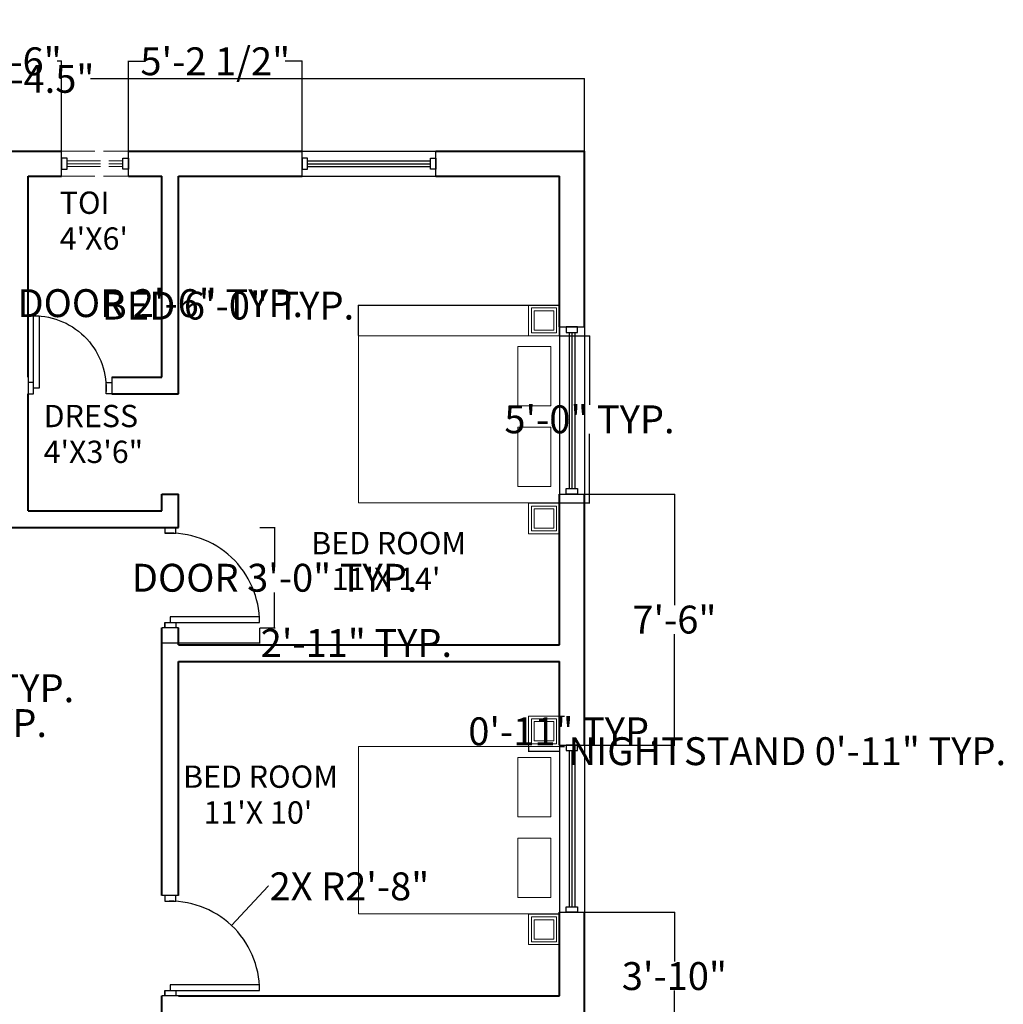
# Model space of a CAD drawing. Units: inches. Extents: x -413 to 212, y 1694 to 2633.
# Tile 5 of 5: x -141 to 212, y 2279 to 2633. Entities that reach past the tile are written whole.
import ezdxf

# ---------------------------------------------------------------- set-up
doc = ezdxf.new("R2010")
doc.units = ezdxf.units.IN
doc.header["$MEASUREMENT"] = 0
doc.linetypes.add('ACAD_ISO02W100', pattern=[15, 12, -3])
for name, color, linetype, lineweight in [('A-ANNO-DIMS', 5, 'Continuous', 18), ('A-AREA-IDEN', 251, 'Continuous', 25), ('A-GLAZ-OVHD', 2, 'ACAD_ISO02W100', 18), ('A-GLAZ-VENT', 2, 'Continuous', 25), ('door', 4, 'Continuous', 25), ('furniture', 1, 'Continuous', 18), ('wall', 20, 'Continuous', 40), ('window', 6, 'Continuous', 25)]:
    doc.layers.add(name, color=color, linetype=linetype, lineweight=lineweight)
doc.styles.get("Standard").update_dxf_attribs({"font": 'arial.ttf'})
doc.dimstyles.get("Standard").update_dxf_attribs({"dimtxt": 10, "dimasz": 0.18, "dimexe": 0.18, "dimexo": 0.0625, "dimgap": 0.09, "dimtad": 0, "dimtih": 1, "dimtoh": 1, "dimdec": 1, "dimzin": 0, "dimdsep": 46, "dimlunit": 3, "dimtxsty": 'Standard', "dimblk": 'ARCHTICK', "dimcen": 0.09, "dimadec": 0, "dimazin": 0, "dimtfac": 1, "dimtdec": 1, "dimtofl": 0, "dimtmove": 0, "dimatfit": 3, "dimfxl": 1, "dimtolj": 1, "dimtzin": 0, "dimarcsym": 0})

# ---------------------------------------------------------------- blocks, each defined once
blk = doc.blocks.new('_ArchTick')
at = {"color": 0, "linetype": 'ByBlock', "const_width": 0.15}
blk.add_lwpolyline([(-0.5, -0.5), (0.5, 0.5)], dxfattribs=at)
blk = doc.blocks.new('*D3')
at = {"layer": 'A-ANNO-DIMS', "color": 0, "lineweight": -2, "transparency": 16777216}
for p, q in [((-338.98, 2585.55), (-338.98, 2611.61)), ((-338.98, 2611.43), (-161.81, 2611.43)), ((61.52, 2611.43), (-115.64, 2611.43)), ((61.52, 2585.55), (61.52, 2611.61))]:
    blk.add_line(p, q, dxfattribs=at)
at = {"layer": 'Defpoints', "color": 0, "transparency": 16777216}
for p in [(61.52, 2611.43), (-338.98, 2585.48), (61.52, 2585.48)]:
    blk.add_point(p, dxfattribs=at)
at = {"layer": 'A-ANNO-DIMS', "color": 0, "lineweight": -2, "transparency": 16777216, "xscale": 0.18, "yscale": 0.18, "zscale": 0.18, "rotation": 180}
blk.add_blockref('_ArchTick', (-338.98, 2611.43), dxfattribs=at)
at = {"layer": 'A-ANNO-DIMS', "color": 0, "lineweight": -2, "transparency": 16777216, "xscale": 0.18, "yscale": 0.18, "zscale": 0.18}
blk.add_blockref('_ArchTick', (61.52, 2611.43), dxfattribs=at)
at = {"layer": 'A-ANNO-DIMS', "color": 0, "transparency": 16777216, "insert": (-138.73, 2611.43), "char_height": 10, "attachment_point": 5}
blk.add_mtext('\\A1;33\'-4.5"', dxfattribs=at)
blk = doc.blocks.new('WINDOW-48IN')
for p, q in [((0, 0), (0, 9)), ((0, 9), (48, 9)), ((48, 0), (48, 9)), ((2, 5.5), (46, 5.5)), ((2, 4.5), (46, 4.5)), ((2, 3.5), (46, 3.5)), ((0, 0), (48, 0))]:
    blk.add_line(p, q)
for points in [[(0, 2.5), (2, 2.5), (2, 6.5), (0, 6.5)], [(48, 2.5), (46, 2.5), (46, 6.5), (48, 6.5)]]:
    blk.add_lwpolyline(points, close=True)
blk = doc.blocks.new('WINDOW-60IN')
for p, q in [((0, 60), (9, 60)), ((0, 60), (0, 0)), ((3.5, 58), (3.5, 2)), ((4.5, 58), (4.5, 2)), ((5.5, 58), (5.5, 2)), ((9, 60), (9, 0)), ((0, 0), (9, 0))]:
    blk.add_line(p, q)
for points in [[(2.5, 60), (2.5, 58), (6.5, 58), (6.5, 60)], [(2.5, 0), (2.5, 2), (6.5, 2), (6.5, 0)]]:
    blk.add_lwpolyline(points, close=True)
blk = doc.blocks.new('VENT-JAMBS-24IN')
for p, q in [((0, 0), (0, 9)), ((24, 0), (24, 9))]:
    blk.add_line(p, q)
for points in [[(0, 2.5), (2, 2.5), (2, 6.5), (0, 6.5)], [(24, 2.5), (22, 2.5), (22, 6.5), (24, 6.5)]]:
    blk.add_lwpolyline(points, close=True)
blk = doc.blocks.new('VENT-PANEL-24IN')
for p, q in [((0, 9), (24, 9)), ((2, 5.5), (22, 5.5)), ((2, 4.5), (22, 4.5)), ((2, 3.5), (22, 3.5)), ((0, 0), (24, 0))]:
    blk.add_line(p, q)
blk = doc.blocks.new('DOOR-SWING-36IN')
for p, q in [((3, 34), (-3, 34)), ((3, -2), (-3, -2))]:
    blk.add_line(p, q)
for points in [[(-2, 34), (-2, 32), (2, 32), (2, 34)], [(-2, -2), (-2, 0), (2, 0), (2, -2)], [(0, 0), (32, 0), (32, 2), (0, 2)]]:
    blk.add_lwpolyline(points, close=True)
blk.add_arc((0, 0), 32, 0, 93.5833)
blk = doc.blocks.new('DOOR-SWING-30IN')
for points in [[(0, 0), (0, 26), (-2, 26), (-2, 0)], [(-28, -2), (-26, -2), (-26, 2), (-28, 2)], [(2, -2), (0, -2), (0, 2), (2, 2)]]:
    blk.add_lwpolyline(points, close=True)
blk.add_arc((0, 0), 26, 90, 184.4117)
blk = doc.blocks.new('BED-DOUBLE-60X72')
for p, q in [((0, 60), (72, 60)), ((72, 0), (72, 60)), ((0, 0), (72, 0))]:
    blk.add_line(p, q)
for points in [[(3.06, 34.82), (14.86, 34.82), (14.86, 56.09), (3.06, 56.09)], [(3.06, 5.88), (14.86, 5.88), (14.86, 27.14), (3.06, 27.14)]]:
    blk.add_lwpolyline(points, close=True)
blk = doc.blocks.new('NIGHTSTAND-INSET')
for points in [[(11.05, 0), (0, 0), (0, 10.95), (11.05, 10.95)], [(11.05, 0), (0, 0), (0, 10.95), (11.05, 10.95)], [(10.05, 1), (1, 1), (1, 9.95), (10.05, 9.95)], [(9.05, 2), (2, 2), (2, 8.95), (9.05, 8.95)]]:
    blk.add_lwpolyline(points, close=True)
blk = doc.blocks.new('*D33')
at = {"layer": 'A-ANNO-DIMS', "color": 0, "lineweight": -2, "transparency": 16777216}
for p, q in [((-191.91, 2402.48), (-188.91, 2402.48)), ((-189.09, 2402.48), (-189.09, 2397.98)), ((-189.09, 2383.24), (-189.09, 2387.75)), ((-191.91, 2383.24), (-188.91, 2383.24))]:
    blk.add_line(p, q, dxfattribs=at)
at = {"layer": 'Defpoints', "color": 0, "transparency": 16777216}
for p in [(-191.98, 2402.48), (-189.09, 2402.48), (-191.98, 2383.24)]:
    blk.add_point(p, dxfattribs=at)
at = {"layer": 'A-ANNO-DIMS', "color": 0, "lineweight": -2, "transparency": 16777216, "xscale": 0.18, "yscale": 0.18, "zscale": 0.18}
for p, rotation in [((-189.09, 2402.48), 90), ((-189.09, 2383.24), 270)]:
    blk.add_blockref('_ArchTick', p, dxfattribs=dict(at, rotation=rotation))
at = {"layer": 'A-ANNO-DIMS', "color": 0, "transparency": 16777216, "insert": (-189.09, 2392.86), "char_height": 10, "attachment_point": 5}
blk.add_mtext('\\A1;END TABLE 1\'-7" TYP.', dxfattribs=at)
blk = doc.blocks.new('*D34')
at = {"layer": 'A-ANNO-DIMS', "color": 0, "lineweight": -2, "transparency": 16777216}
for p, q in [((-208.77, 2383.18), (-208.77, 2380.17)), ((-208.77, 2380.35), (-191.98, 2380.35)), ((-191.98, 2383.18), (-191.98, 2380.17)), ((-191.98, 2380.35), (-191.8, 2380.35))]:
    blk.add_line(p, q, dxfattribs=at)
at = {"layer": 'Defpoints', "color": 0, "transparency": 16777216}
for p in [(-208.77, 2383.24), (-191.98, 2383.24), (-191.98, 2380.35)]:
    blk.add_point(p, dxfattribs=at)
at = {"layer": 'A-ANNO-DIMS', "color": 0, "lineweight": -2, "transparency": 16777216, "xscale": 0.18, "yscale": 0.18, "zscale": 0.18, "rotation": 180}
blk.add_blockref('_ArchTick', (-208.77, 2380.35), dxfattribs=at)
at = {"layer": 'A-ANNO-DIMS', "color": 0, "lineweight": -2, "transparency": 16777216, "xscale": 0.18, "yscale": 0.18, "zscale": 0.18}
blk.add_blockref('_ArchTick', (-191.98, 2380.35), dxfattribs=at)
at = {"layer": 'A-ANNO-DIMS', "color": 0, "transparency": 16777216, "insert": (-161.7, 2380.35), "char_height": 10, "attachment_point": 5}
blk.add_mtext('\\A1;1\'-5" TYP.', dxfattribs=at)
blk = doc.blocks.new('*D35')
at = {"layer": 'A-ANNO-DIMS', "color": 0, "lineweight": -2, "transparency": 16777216}
for p, q in [((-173.98, 2526.55), (-173.98, 2531.16)), ((-173.98, 2530.98), (-143.98, 2530.98)), ((-143.98, 2526.55), (-143.98, 2531.16)), ((-143.98, 2530.98), (-143.8, 2530.98))]:
    blk.add_line(p, q, dxfattribs=at)
at = {"layer": 'Defpoints', "color": 0, "transparency": 16777216}
for p in [(-143.98, 2530.98), (-173.98, 2526.48), (-143.98, 2526.48)]:
    blk.add_point(p, dxfattribs=at)
at = {"layer": 'A-ANNO-DIMS', "color": 0, "lineweight": -2, "transparency": 16777216, "xscale": 0.18, "yscale": 0.18, "zscale": 0.18, "rotation": 180}
blk.add_blockref('_ArchTick', (-173.98, 2530.98), dxfattribs=at)
at = {"layer": 'A-ANNO-DIMS', "color": 0, "lineweight": -2, "transparency": 16777216, "xscale": 0.18, "yscale": 0.18, "zscale": 0.18}
blk.add_blockref('_ArchTick', (-143.98, 2530.98), dxfattribs=at)
at = {"layer": 'A-ANNO-DIMS', "color": 0, "transparency": 16777216, "insert": (-90.58, 2530.98), "char_height": 10, "attachment_point": 5}
blk.add_mtext('\\A1;DOOR 2\'-6" TYP.', dxfattribs=at)
blk = doc.blocks.new('*D37')
at = {"layer": 'A-ANNO-DIMS', "color": 0, "lineweight": -2, "transparency": 16777216}
for p, q in [((-54.91, 2450.48), (-49.4, 2450.48)), ((-49.58, 2450.48), (-49.58, 2437.75)), ((-49.58, 2414.48), (-49.58, 2427.22)), ((-54.91, 2414.48), (-49.4, 2414.48))]:
    blk.add_line(p, q, dxfattribs=at)
at = {"layer": 'Defpoints', "color": 0, "transparency": 16777216}
for p in [(-54.98, 2450.48), (-49.58, 2450.48), (-54.98, 2414.48)]:
    blk.add_point(p, dxfattribs=at)
at = {"layer": 'A-ANNO-DIMS', "color": 0, "lineweight": -2, "transparency": 16777216, "xscale": 0.18, "yscale": 0.18, "zscale": 0.18}
for p, rotation in [((-49.58, 2450.48), 90), ((-49.58, 2414.48), 270)]:
    blk.add_blockref('_ArchTick', p, dxfattribs=dict(at, rotation=rotation))
at = {"layer": 'A-ANNO-DIMS', "color": 0, "transparency": 16777216, "insert": (-49.58, 2432.48), "char_height": 10, "attachment_point": 5}
blk.add_mtext('\\A1;DOOR 3\'-0" TYP.', dxfattribs=at)
blk = doc.blocks.new('*D38')
at = {"layer": 'A-ANNO-DIMS', "color": 0, "lineweight": -2, "transparency": 16777216}
for p, q in [((-89.98, 2414.42), (-89.98, 2408.9)), ((-54.98, 2414.42), (-54.98, 2408.9)), ((-89.98, 2409.08), (-54.98, 2409.08)), ((-54.98, 2409.08), (-54.8, 2409.08))]:
    blk.add_line(p, q, dxfattribs=at)
at = {"layer": 'Defpoints', "color": 0, "transparency": 16777216}
for p in [(-89.98, 2414.48), (-54.98, 2414.48), (-54.98, 2409.08)]:
    blk.add_point(p, dxfattribs=at)
at = {"layer": 'A-ANNO-DIMS', "color": 0, "lineweight": -2, "transparency": 16777216, "xscale": 0.18, "yscale": 0.18, "zscale": 0.18, "rotation": 180}
blk.add_blockref('_ArchTick', (-89.98, 2409.08), dxfattribs=at)
at = {"layer": 'A-ANNO-DIMS', "color": 0, "lineweight": -2, "transparency": 16777216, "xscale": 0.18, "yscale": 0.18, "zscale": 0.18}
blk.add_blockref('_ArchTick', (-54.98, 2409.08), dxfattribs=at)
at = {"layer": 'A-ANNO-DIMS', "color": 0, "transparency": 16777216, "insert": (-20.26, 2409.08), "char_height": 10, "attachment_point": 5}
blk.add_mtext('\\A1;2\'-11" TYP.', dxfattribs=at)
blk = doc.blocks.new('*D39')
at = {"layer": 'A-ANNO-DIMS', "color": 0, "lineweight": -2, "transparency": 16777216}
for p, q in [((-19.48, 2530.1), (-19.66, 2530.1)), ((-19.48, 2519.36), (-19.48, 2530.28)), ((52.52, 2530.1), (-19.48, 2530.1)), ((52.52, 2519.36), (52.52, 2530.28))]:
    blk.add_line(p, q, dxfattribs=at)
at = {"layer": 'Defpoints', "color": 0, "transparency": 16777216}
for p in [(-19.48, 2530.1), (-19.48, 2519.3), (52.52, 2519.3)]:
    blk.add_point(p, dxfattribs=at)
at = {"layer": 'A-ANNO-DIMS', "color": 0, "lineweight": -2, "transparency": 16777216, "xscale": 0.18, "yscale": 0.18, "zscale": 0.18, "rotation": 180}
blk.add_blockref('_ArchTick', (-19.48, 2530.1), dxfattribs=at)
at = {"layer": 'A-ANNO-DIMS', "color": 0, "lineweight": -2, "transparency": 16777216, "xscale": 0.18, "yscale": 0.18, "zscale": 0.18}
blk.add_blockref('_ArchTick', (52.52, 2530.1), dxfattribs=at)
at = {"layer": 'A-ANNO-DIMS', "color": 0, "transparency": 16777216, "insert": (-66.3, 2530.1), "char_height": 10, "attachment_point": 5}
blk.add_mtext('\\A1;BED 6\'-0" TYP.', dxfattribs=at)
blk = doc.blocks.new('*D40')
at = {"layer": 'A-ANNO-DIMS', "color": 0, "lineweight": -2, "transparency": 16777216}
for p, q in [((52.59, 2519.3), (63.5, 2519.3)), ((63.32, 2519.3), (63.32, 2494.5)), ((63.32, 2459.3), (63.32, 2484.1)), ((52.59, 2459.3), (63.5, 2459.3))]:
    blk.add_line(p, q, dxfattribs=at)
at = {"layer": 'Defpoints', "color": 0, "transparency": 16777216}
for p in [(52.52, 2519.3), (63.32, 2519.3), (52.52, 2459.3)]:
    blk.add_point(p, dxfattribs=at)
at = {"layer": 'A-ANNO-DIMS', "color": 0, "lineweight": -2, "transparency": 16777216, "xscale": 0.18, "yscale": 0.18, "zscale": 0.18}
for p, rotation in [((63.32, 2519.3), 90), ((63.32, 2459.3), 270)]:
    blk.add_blockref('_ArchTick', p, dxfattribs=dict(at, rotation=rotation))
at = {"layer": 'A-ANNO-DIMS', "color": 0, "transparency": 16777216, "insert": (63.32, 2489.3), "char_height": 10, "attachment_point": 5}
blk.add_mtext('\\A1;5\'-0" TYP.', dxfattribs=at)
blk = doc.blocks.new('*D41')
at = {"layer": 'A-ANNO-DIMS', "color": 0, "lineweight": -2, "transparency": 16777216}
for p, q in [((41.48, 2371.86), (41.48, 2370.09)), ((41.48, 2370.27), (52.52, 2370.27)), ((52.52, 2371.86), (52.52, 2370.09)), ((52.52, 2370.27), (52.7, 2370.27))]:
    blk.add_line(p, q, dxfattribs=at)
at = {"layer": 'Defpoints', "color": 0, "transparency": 16777216}
for p in [(41.48, 2371.93), (52.52, 2371.93), (52.52, 2370.27)]:
    blk.add_point(p, dxfattribs=at)
at = {"layer": 'A-ANNO-DIMS', "color": 0, "lineweight": -2, "transparency": 16777216, "xscale": 0.18, "yscale": 0.18, "zscale": 0.18, "rotation": 180}
blk.add_blockref('_ArchTick', (41.48, 2370.27), dxfattribs=at)
at = {"layer": 'A-ANNO-DIMS', "color": 0, "lineweight": -2, "transparency": 16777216, "xscale": 0.18, "yscale": 0.18, "zscale": 0.18}
blk.add_blockref('_ArchTick', (52.52, 2370.27), dxfattribs=at)
at = {"layer": 'A-ANNO-DIMS', "color": 0, "transparency": 16777216, "insert": (134.26, 2370.27), "char_height": 10, "attachment_point": 5}
blk.add_mtext('\\A1;NIGHTSTAND 0\'-11" TYP.', dxfattribs=at)
blk = doc.blocks.new('*D42')
at = {"layer": 'A-ANNO-DIMS', "color": 0, "lineweight": -2, "transparency": 16777216}
for p, q in [((52.59, 2382.87), (54.36, 2382.87)), ((54.18, 2382.87), (54.18, 2382.6)), ((52.59, 2371.93), (54.36, 2371.93)), ((54.18, 2371.93), (54.18, 2372.2))]:
    blk.add_line(p, q, dxfattribs=at)
at = {"layer": 'Defpoints', "color": 0, "transparency": 16777216}
for p in [(52.52, 2382.87), (54.18, 2382.87), (52.52, 2371.93)]:
    blk.add_point(p, dxfattribs=at)
at = {"layer": 'A-ANNO-DIMS', "color": 0, "lineweight": -2, "transparency": 16777216, "xscale": 0.18, "yscale": 0.18, "zscale": 0.18}
for p, rotation in [((54.18, 2382.87), 90), ((54.18, 2371.93), 270)]:
    blk.add_blockref('_ArchTick', p, dxfattribs=dict(at, rotation=rotation))
at = {"layer": 'A-ANNO-DIMS', "color": 0, "transparency": 16777216, "insert": (54.18, 2377.4), "char_height": 10, "attachment_point": 5}
blk.add_mtext('\\A1;0\'-11" TYP.', dxfattribs=at)
blk = doc.blocks.new('*D66')
at = {"layer": 'A-ANNO-DIMS', "color": 0, "lineweight": -2, "transparency": 16777216}
for p, q in [((-155.98, 2585.55), (-155.98, 2617.91)), ((-155.98, 2617.73), (-154.44, 2617.73)), ((-125.98, 2617.73), (-127.51, 2617.73)), ((-125.98, 2585.55), (-125.98, 2617.91))]:
    blk.add_line(p, q, dxfattribs=at)
at = {"layer": 'Defpoints', "color": 0, "transparency": 16777216}
for p in [(-125.98, 2617.73), (-155.98, 2585.48), (-125.98, 2585.48)]:
    blk.add_point(p, dxfattribs=at)
at = {"layer": 'A-ANNO-DIMS', "color": 0, "lineweight": -2, "transparency": 16777216, "xscale": 0.18, "yscale": 0.18, "zscale": 0.18, "rotation": 180}
blk.add_blockref('_ArchTick', (-155.98, 2617.73), dxfattribs=at)
at = {"layer": 'A-ANNO-DIMS', "color": 0, "lineweight": -2, "transparency": 16777216, "xscale": 0.18, "yscale": 0.18, "zscale": 0.18}
blk.add_blockref('_ArchTick', (-125.98, 2617.73), dxfattribs=at)
at = {"layer": 'A-ANNO-DIMS', "color": 0, "transparency": 16777216, "insert": (-140.98, 2617.73), "char_height": 10, "attachment_point": 5}
blk.add_mtext('\\A1;2\'-6"', dxfattribs=at)
blk = doc.blocks.new('*D67')
at = {"layer": 'A-ANNO-DIMS', "color": 0, "lineweight": -2, "transparency": 16777216}
for p, q in [((-101.98, 2585.55), (-101.98, 2617.91)), ((-101.98, 2617.73), (-95.88, 2617.73)), ((-39.73, 2617.73), (-45.82, 2617.73)), ((-39.73, 2585.55), (-39.73, 2617.91))]:
    blk.add_line(p, q, dxfattribs=at)
at = {"layer": 'Defpoints', "color": 0, "transparency": 16777216}
for p in [(-39.73, 2617.73), (-101.98, 2585.48), (-39.73, 2585.48)]:
    blk.add_point(p, dxfattribs=at)
at = {"layer": 'A-ANNO-DIMS', "color": 0, "lineweight": -2, "transparency": 16777216, "xscale": 0.18, "yscale": 0.18, "zscale": 0.18, "rotation": 180}
blk.add_blockref('_ArchTick', (-101.98, 2617.73), dxfattribs=at)
at = {"layer": 'A-ANNO-DIMS', "color": 0, "lineweight": -2, "transparency": 16777216, "xscale": 0.18, "yscale": 0.18, "zscale": 0.18}
blk.add_blockref('_ArchTick', (-39.73, 2617.73), dxfattribs=at)
at = {"layer": 'A-ANNO-DIMS', "color": 0, "transparency": 16777216, "insert": (-70.85, 2617.73), "char_height": 10, "attachment_point": 5}
blk.add_mtext('\\A1;5\'-2 1/2"', dxfattribs=at)
blk = doc.blocks.new('*D71')
at = {"layer": 'A-ANNO-DIMS', "color": 0, "lineweight": -2, "transparency": 16777216}
for p, q in [((61.59, 2462.48), (93.95, 2462.48)), ((93.77, 2462.48), (93.77, 2422.68)), ((93.77, 2372.48), (93.77, 2412.29)), ((61.59, 2372.48), (93.95, 2372.48))]:
    blk.add_line(p, q, dxfattribs=at)
at = {"layer": 'Defpoints', "color": 0, "transparency": 16777216}
for p in [(61.52, 2462.48), (61.52, 2372.48), (93.77, 2372.48)]:
    blk.add_point(p, dxfattribs=at)
at = {"layer": 'A-ANNO-DIMS', "color": 0, "lineweight": -2, "transparency": 16777216, "xscale": 0.18, "yscale": 0.18, "zscale": 0.18}
for p, rotation in [((93.77, 2462.48), 90), ((93.77, 2372.48), 270)]:
    blk.add_blockref('_ArchTick', p, dxfattribs=dict(at, rotation=rotation))
at = {"layer": 'A-ANNO-DIMS', "color": 0, "transparency": 16777216, "insert": (93.77, 2417.48), "char_height": 10, "attachment_point": 5}
blk.add_mtext('\\A1;7\'-6"', dxfattribs=at)
blk = doc.blocks.new('*D72')
at = {"layer": 'A-ANNO-DIMS', "color": 0, "lineweight": -2, "transparency": 16777216}
for p, q in [((61.59, 2312.48), (93.95, 2312.48)), ((93.77, 2312.48), (93.77, 2294.81)), ((93.77, 2266.73), (93.77, 2284.41)), ((61.59, 2266.73), (93.95, 2266.73))]:
    blk.add_line(p, q, dxfattribs=at)
at = {"layer": 'Defpoints', "color": 0, "transparency": 16777216}
for p in [(61.52, 2312.48), (61.52, 2266.73), (93.77, 2266.73)]:
    blk.add_point(p, dxfattribs=at)
at = {"layer": 'A-ANNO-DIMS', "color": 0, "lineweight": -2, "transparency": 16777216, "xscale": 0.18, "yscale": 0.18, "zscale": 0.18}
for p, rotation in [((93.77, 2312.48), 90), ((93.77, 2266.73), 270)]:
    blk.add_blockref('_ArchTick', p, dxfattribs=dict(at, rotation=rotation))
at = {"layer": 'A-ANNO-DIMS', "color": 0, "transparency": 16777216, "insert": (93.77, 2289.61), "char_height": 10, "attachment_point": 5}
blk.add_mtext('\\A1;3\'-10"', dxfattribs=at)
blk = doc.blocks.new('*D83')
at = {"layer": 'A-ANNO-DIMS', "color": 0, "lineweight": -2, "transparency": 16777216}
for p, q in [((-51.92, 2321.8), (-65.07, 2307.81)), ((-51.74, 2321.8), (-51.92, 2321.8)), ((-87.07, 2284.48), (-86.89, 2284.48)), ((-86.98, 2284.39), (-86.98, 2284.57))]:
    blk.add_line(p, q, dxfattribs=at)
at = {"layer": 'Defpoints', "color": 0, "transparency": 16777216}
for p in [(-65.07, 2307.81), (-86.98, 2284.48)]:
    blk.add_point(p, dxfattribs=at)
at = {"layer": 'A-ANNO-DIMS', "color": 0, "lineweight": -2, "transparency": 16777216, "xscale": 0.18, "yscale": 0.18, "zscale": 0.18, "rotation": 226.7915046823963}
blk.add_blockref('_ArchTick', (-65.07, 2307.81), dxfattribs=at)
at = {"layer": 'A-ANNO-DIMS', "color": 0, "transparency": 16777216, "insert": (-22.75, 2321.8), "char_height": 10, "attachment_point": 5}
blk.add_mtext('\\A1;2X R2\'-8"', dxfattribs=at)

msp = doc.modelspace()

# ---------------------------------------------------------------- linework, layer by layer
at = {"layer": 'door'}
for p, q in [((-137.98, 2504.48), (-137.98, 2498.48)), ((-107.98, 2504.48), (-107.98, 2498.48)), ((-88.98, 2450.48), (-88.98, 2448.42)), ((-88.98, 2416.48), (-88.98, 2414.48)), ((-88.98, 2318.48), (-88.98, 2316.42)), ((-88.98, 2284.48), (-88.98, 2282.48))]:
    msp.add_line(p, q, dxfattribs=at)
at = {"layer": 'wall'}
for p, q in [((-155.98, 2585.48), (-125.98, 2585.48)), ((-101.98, 2585.48), (-39.73, 2585.48)), ((8.27, 2585.48), (61.52, 2585.48)), ((61.52, 2522.48), (61.52, 2585.48)), ((-137.98, 2576.48), (-125.98, 2576.48)), ((-137.98, 2504.48), (-137.98, 2576.48)), ((-101.98, 2576.48), (-89.98, 2576.48)), ((-89.98, 2504.48), (-89.98, 2576.48)), ((-83.98, 2498.48), (-83.98, 2576.48)), ((-83.98, 2576.48), (-39.73, 2576.48)), ((8.27, 2576.48), (52.52, 2576.48)), ((52.52, 2522.48), (52.52, 2576.48)), ((-107.98, 2504.48), (-89.98, 2504.48)), ((-137.98, 2456.48), (-137.98, 2498.48)), ((-107.98, 2498.48), (-83.98, 2498.48)), ((-89.98, 2462.48), (-83.98, 2462.48)), ((-89.98, 2456.48), (-89.98, 2462.48)), ((-83.98, 2450.48), (-83.98, 2462.48)), ((52.52, 2408.48), (52.52, 2462.48)), ((61.52, 2372.48), (61.52, 2462.48)), ((-137.98, 2456.48), (-89.98, 2456.48)), ((-197.98, 2450.48), (-83.98, 2450.48)), ((-89.98, 2402.48), (-89.98, 2414.48)), ((-83.98, 2408.48), (-83.98, 2414.48)), ((-83.98, 2408.48), (52.52, 2408.48)), ((-89.98, 2318.48), (-89.98, 2402.48)), ((-83.98, 2402.48), (52.52, 2402.48)), ((-83.98, 2318.48), (-83.98, 2402.48)), ((52.52, 2372.48), (52.52, 2402.48)), ((52.52, 2282.48), (52.52, 2312.48)), ((61.52, 2266.73), (61.52, 2312.48)), ((-89.98, 2276.48), (-89.98, 2282.48)), ((-83.98, 2282.48), (52.52, 2282.48))]:
    msp.add_line(p, q, dxfattribs=at)

# ---------------------------------------------------------------- block references
at = {"layer": 'A-GLAZ-OVHD'}
msp.add_blockref('VENT-PANEL-24IN', (-125.98, 2576.49), dxfattribs=at)
at = {"layer": 'A-GLAZ-VENT'}
msp.add_blockref('VENT-JAMBS-24IN', (-125.98, 2576.49), dxfattribs=at)
at = {"layer": 'door', "extrusion": (0, 0, -1), "zscale": -1}
msp.add_blockref('DOOR-SWING-30IN', (135.98, 2500.48), dxfattribs=at)
at = {"layer": 'door'}
for p in [(-86.98, 2416.48), (-86.98, 2284.48)]:
    msp.add_blockref('DOOR-SWING-36IN', p, dxfattribs=at)
at = {"layer": 'furniture'}
for p in [(41.48, 2519.3), (41.48, 2448.26), (41.48, 2371.93), (41.48, 2300.88)]:
    msp.add_blockref('NIGHTSTAND-INSET', p, dxfattribs=at)
at = {"layer": 'furniture', "extrusion": (0, 0, -1), "zscale": -1}
for p in [(-52.52, 2459.3), (-52.52, 2311.93)]:
    msp.add_blockref('BED-DOUBLE-60X72', p, dxfattribs=at)
at = {"layer": 'window'}
for name, p in [('WINDOW-48IN', (-39.73, 2576.49)), ('WINDOW-60IN', (52.52, 2462.49)), ('WINDOW-60IN', (52.52, 2312.49))]:
    msp.add_blockref(name, p, dxfattribs=at)

# ---------------------------------------------------------------- texts
at = {"layer": 'A-AREA-IDEN'}
for s, p in [('TOI', (-126.61, 2563)), ("4'X6'", (-126.61, 2550.15)), ('DRESS ', (-132.39, 2486.49)), ('4\'X3\'6"', (-132.39, 2473.64)), ('BED ROOM ', (-36.45, 2440.91)), ("   11'X 14'", (-36.45, 2428.06)), ('BED ROOM ', (-82.4, 2357.14)), ("   11'X 10'", (-82.4, 2344.29))]:
    msp.add_text(s, height=8, dxfattribs=at).set_placement(p)

# ---------------------------------------------------------------- dimensions: what is measured, and where the dimension line sits
at = {"layer": 'A-ANNO-DIMS'}
for base, p1, p2, override, picture, middle in [((-39.725666, 2617.734571), (-101.975666, 2585.484571), (-39.725666, 2585.484571), {"dimdec": 1, "dimlfac": 1, "dimrnd": 0, "dimzin": 1, "dimdsep": 46, "dimlunit": 4, "dimfrac": 2}, '*D67', (-70.850666, 2617.734571)), ((-125.98, 2617.73), (-155.98, 2585.48), (-125.98, 2585.48), {"dimdec": 1, "dimlfac": 1, "dimrnd": 0, "dimzin": 1, "dimdsep": 46, "dimlunit": 4, "dimfrac": 2}, '*D66', (-140.98, 2617.73)), ((61.52, 2611.43), (-338.98, 2585.48), (61.52, 2585.48), {"dimclrd": 0, "dimclre": 0, "dimclrt": 0}, '*D3', (-138.73, 2611.43))]:
    dim = msp.add_linear_dim(base=base, p1=p1, p2=p2, dimstyle='Standard', override=override, dxfattribs=at)
    dim.commit()
    dim.dimension.update_dxf_attribs({"geometry": picture, "text_midpoint": middle})
for base, p1, p2, text, picture, middle in [((-143.98, 2530.98), (-173.98, 2526.48), (-143.98, 2526.48), 'DOOR <> TYP.', '*D35', (-90.58, 2530.98)), ((-54.98, 2409.08), (-89.98, 2414.48), (-54.98, 2414.48), '<> TYP.', '*D38', (-20.26, 2409.08)), ((-191.98, 2380.35), (-208.77, 2383.24), (-191.98, 2383.24), '<> TYP.', '*D34', (-161.7, 2380.35)), ((52.52, 2370.27), (41.48, 2371.93), (52.52, 2371.93), 'NIGHTSTAND <> TYP.', '*D41', (134.26, 2370.27))]:
    dim = msp.add_linear_dim(base=base, p1=p1, p2=p2, text=text, dimstyle='Standard', override={"dimdec": 1, "dimlfac": 1, "dimrnd": 0, "dimzin": 1, "dimdsep": 46, "dimlunit": 4, "dimfrac": 2}, dxfattribs=at)
    dim.commit()
    dim.dimension.update_dxf_attribs({"geometry": picture, "text_midpoint": middle})
for base, p1, p2, angle, text, picture, middle in [((-19.48, 2530.1), (52.52, 2519.3), (-19.48, 2519.3), 180, 'BED <> TYP.', '*D39', (-66.3, 2530.1)), ((63.32, 2519.3), (52.52, 2459.3), (52.52, 2519.3), 90, '<> TYP.', '*D40', (63.32, 2489.3)), ((-49.58, 2450.48), (-54.98, 2414.48), (-54.98, 2450.48), 90, 'DOOR <> TYP.', '*D37', (-49.58, 2432.48)), ((-189.09, 2402.48), (-191.98, 2383.24), (-191.98, 2402.48), 90, 'END TABLE <> TYP.', '*D33', (-189.09, 2392.86)), ((54.18, 2382.87), (52.52, 2371.93), (52.52, 2382.87), 90, '<> TYP.', '*D42', (54.18, 2377.4))]:
    dim = msp.add_linear_dim(base=base, p1=p1, p2=p2, angle=angle, text=text, dimstyle='Standard', override={"dimdec": 1, "dimlfac": 1, "dimrnd": 0, "dimzin": 1, "dimdsep": 46, "dimlunit": 4, "dimfrac": 2}, dxfattribs=at)
    dim.commit()
    dim.dimension.update_dxf_attribs({"geometry": picture, "text_midpoint": middle})
for base, p1, p2, picture, middle in [((93.77, 2372.48), (61.52, 2462.48), (61.52, 2372.48), '*D71', (93.77, 2417.48)), ((93.774334, 2266.734571), (61.524334, 2312.484571), (61.524334, 2266.734571), '*D72', (93.774334, 2289.609571))]:
    dim = msp.add_linear_dim(base=base, p1=p1, p2=p2, angle=90, dimstyle='Standard', override={"dimdec": 1, "dimlfac": 1, "dimrnd": 0, "dimzin": 1, "dimdsep": 46, "dimlunit": 4, "dimfrac": 2}, dxfattribs=at)
    dim.commit()
    dim.dimension.update_dxf_attribs({"geometry": picture, "text_midpoint": middle})
dim = msp.add_radius_dim(center=(-86.98, 2284.48), mpoint=(-65.07, 2307.81), text='2X <>', dimstyle='Standard', override={"dimdec": 1, "dimlfac": 1, "dimrnd": 0, "dimzin": 1, "dimdsep": 46, "dimlunit": 4, "dimfrac": 2}, dxfattribs=at)
dim.commit()
dim.dimension.update_dxf_attribs({"geometry": '*D83', "text_midpoint": (-22.75, 2321.8), "dimtype": 164})

doc.saveas('drawing.dxf')
